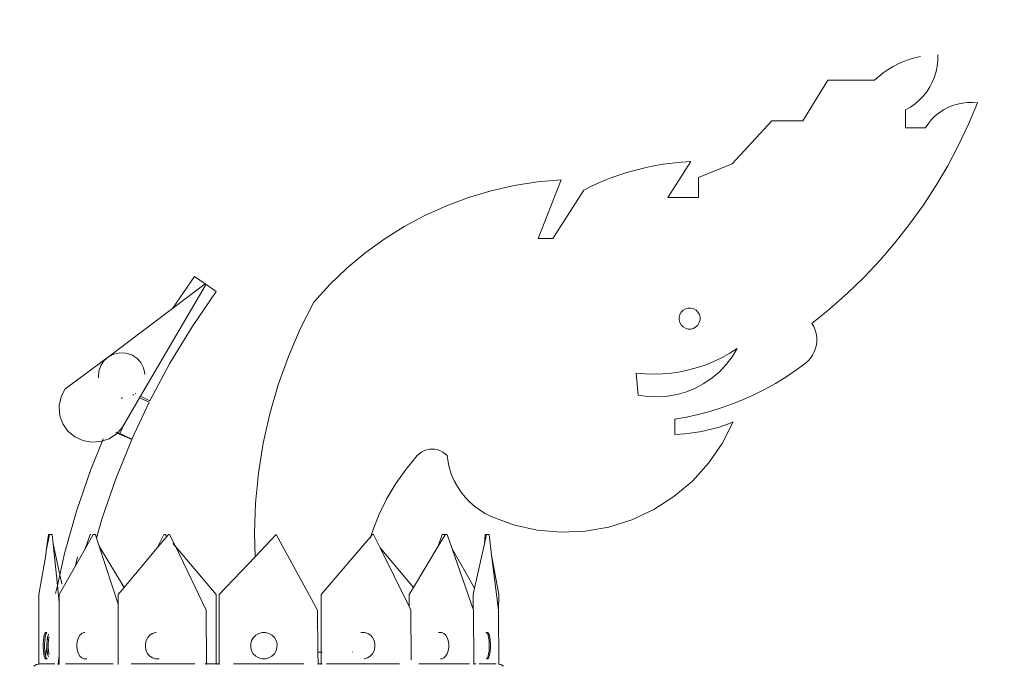
# Model space of a CAD drawing. Units: millimetres. Extents: x 7894 to 8038, y 6851 to 6951.
# Tile 40 of 49: x 7969.515 to 7972.111, y 6926.755 to 6928.457. Entities that reach past the tile are written whole.
import ezdxf

# ---------------------------------------------------------------- set-up
doc = ezdxf.new("R2010")
doc.units = ezdxf.units.MM
doc.layers.add('A-ANNO-DIMS', color=2, linetype='Continuous', lineweight=18)
doc.layers.add('A-FURN-ACCS', color=8, linetype='Continuous', lineweight=13)
doc.styles.get("Standard").update_dxf_attribs({"font": 'arial.ttf'})
doc.dimstyles.new('ISO-25', dxfattribs={"dimtxt": 1, "dimasz": 1, "dimexe": 1.25, "dimexo": 0.625, "dimtad": 1, "dimdec": 0, "dimlunit": 4, "dimtxsty": 'Standard', "dimcen": 2.5, "dimclrt": 1, "dimadec": 0, "dimazin": 0, "dimtfac": 1, "dimtdec": 0, "dimtmove": 0, "dimatfit": 3, "dimfxl": 1, "dimarcsym": 0})

# ---------------------------------------------------------------- blocks, each defined once
blk = doc.blocks.new('DISPLAY-LEAF-FINIAL-Z2_152')
for p, q in [((2.565, 3.5085, 2.1518), (2.5649, 3.4937, 2.1518)), ((2.4472, 3.4779, 2.1518), (2.4609, 3.4849, 2.1518)), ((2.4609, 3.4849, 2.1518), (2.4749, 3.4911, 2.1518)), ((2.4749, 3.4911, 2.1518), (2.4894, 3.4964, 2.1518)), ((2.4894, 3.4964, 2.1518), (2.5041, 3.5007, 2.1518)), ((2.5041, 3.5007, 2.1518), (2.5191, 3.5041, 2.1518)), ((2.5634, 3.479, 2.1518), (2.5605, 3.4646, 2.1518)), ((2.5649, 3.4937, 2.1518), (2.5634, 3.479, 2.1518)), ((2.4094, 3.4516, 2.1518), (2.4214, 3.4612, 2.1518)), ((2.4214, 3.4612, 2.1518), (2.4341, 3.4699, 2.1518)), ((2.4341, 3.4699, 2.1518), (2.4472, 3.4779, 2.1518)), ((2.5605, 3.4646, 2.1518), (2.5562, 3.4504, 2.1518)), ((2.2094, 3.3343, 2.1518), (2.2756, 3.4413, 2.1518)), ((2.2756, 3.4413, 2.1518), (2.3979, 3.4413, 2.1518)), ((2.3979, 3.4413, 2.1518), (2.4094, 3.4516, 2.1518)), ((2.5507, 3.4368, 2.1518), (2.5438, 3.4237, 2.1518)), ((2.5562, 3.4504, 2.1518), (2.5507, 3.4368, 2.1518)), ((2.5358, 3.4113, 2.1518), (2.5266, 3.3997, 2.1518)), ((2.5438, 3.4237, 2.1518), (2.5358, 3.4113, 2.1518)), ((2.5052, 3.3794, 2.1518), (2.4932, 3.3709, 2.1518)), ((2.5164, 3.3891, 2.1518), (2.5052, 3.3794, 2.1518)), ((2.5266, 3.3997, 2.1518), (2.5164, 3.3891, 2.1518)), ((2.5917, 3.3696, 2.1518), (2.604, 3.3748, 2.1518)), ((2.604, 3.3748, 2.1518), (2.6168, 3.3788, 2.1518)), ((2.6168, 3.3788, 2.1518), (2.63, 3.3815, 2.1518)), ((2.63, 3.3815, 2.1518), (2.6433, 3.3829, 2.1518)), ((2.6433, 3.3829, 2.1518), (2.6567, 3.3831, 2.1518)), ((2.6701, 3.3819, 2.1518), (2.6462, 3.3254, 2.1518)), ((2.6567, 3.3831, 2.1518), (2.6701, 3.3819, 2.1518)), ((2.4932, 3.3709, 2.1518), (2.4804, 3.3636, 2.1518)), ((2.4804, 3.3636, 2.1518), (2.4804, 3.3164, 2.1518)), ((2.5584, 3.3473, 2.1518), (2.5687, 3.3558, 2.1518)), ((2.5687, 3.3558, 2.1518), (2.5799, 3.3633, 2.1518)), ((2.5799, 3.3633, 2.1518), (2.5917, 3.3696, 2.1518)), ((2.0233, 3.2209, 2.1518), (2.1272, 3.3343, 2.1518)), ((2.1272, 3.3343, 2.1518), (2.2094, 3.3343, 2.1518)), ((2.5329, 3.3164, 2.1518), (2.5403, 3.3275, 2.1518)), ((2.5403, 3.3275, 2.1518), (2.5489, 3.3378, 2.1518)), ((2.5489, 3.3378, 2.1518), (2.5584, 3.3473, 2.1518)), ((2.6462, 3.3254, 2.1518), (2.6199, 3.27, 2.1518)), ((2.4804, 3.3164, 2.1518), (2.5329, 3.3164, 2.1518)), ((2.6199, 3.27, 2.1518), (2.5912, 3.2159, 2.1518)), ((1.8166, 3.2158, 2.1518), (1.8408, 3.2199, 2.1518)), ((1.8408, 3.2199, 2.1518), (1.8651, 3.2232, 2.1518)), ((1.9139, 3.2271, 2.1518), (1.8536, 3.1329, 2.1518)), ((1.8651, 3.2232, 2.1518), (1.8895, 3.2256, 2.1518)), ((1.8895, 3.2256, 2.1518), (1.9139, 3.2271, 2.1518)), ((1.934, 3.1854, 2.1518), (2.0233, 3.2209, 2.1518)), ((1.7219, 3.1906, 2.1518), (1.7452, 3.1982, 2.1518)), ((1.7452, 3.1982, 2.1518), (1.7688, 3.2049, 2.1518)), ((1.7688, 3.2049, 2.1518), (1.7926, 3.2108, 2.1518)), ((1.7926, 3.2108, 2.1518), (1.8166, 3.2158, 2.1518)), ((2.5912, 3.2159, 2.1518), (2.56, 3.1631, 2.1518)), ((1.4486, 3.1639, 2.1518), (1.5102, 3.1734, 2.1518)), ((1.5102, 3.1734, 2.1518), (1.5723, 3.1787, 2.1518)), ((1.5723, 3.1787, 2.1518), (1.5113, 3.0242, 2.1518)), ((1.6538, 3.163, 2.1518), (1.6762, 3.1731, 2.1518)), ((1.6762, 3.1731, 2.1518), (1.6989, 3.1823, 2.1518)), ((1.6989, 3.1823, 2.1518), (1.7219, 3.1906, 2.1518)), ((1.934, 3.1329, 2.1518), (1.934, 3.1854, 2.1518)), ((1.3281, 3.1326, 2.1518), (1.3879, 3.1503, 2.1518)), ((1.3879, 3.1503, 2.1518), (1.4486, 3.1639, 2.1518)), ((1.5498, 3.0242, 2.1518), (1.6318, 3.1522, 2.1518)), ((1.6318, 3.1522, 2.1518), (1.6538, 3.163, 2.1518)), ((2.56, 3.1631, 2.1518), (2.5265, 3.1117, 2.1518)), ((1.2698, 3.1109, 2.1518), (1.3281, 3.1326, 2.1518)), ((1.8536, 3.1329, 2.1518), (1.934, 3.1329, 2.1518)), ((1.213, 3.0852, 2.1518), (1.2698, 3.1109, 2.1518)), ((2.5265, 3.1117, 2.1518), (2.4908, 3.0619, 2.1518)), ((1.1581, 3.0558, 2.1518), (1.213, 3.0852, 2.1518)), ((1.1053, 3.0227, 2.1518), (1.1581, 3.0558, 2.1518)), ((2.4908, 3.0619, 2.1518), (2.4529, 3.0137, 2.1518)), ((1.0549, 2.9861, 2.1518), (1.1053, 3.0227, 2.1518)), ((1.5113, 3.0242, 2.1518), (1.5498, 3.0242, 2.1518)), ((2.4529, 3.0137, 2.1518), (2.4129, 2.9672, 2.1518)), ((1.0071, 2.9462, 2.1518), (1.0549, 2.9861, 2.1518)), ((2.4129, 2.9672, 2.1518), (2.3708, 2.9226, 2.1518)), ((0.9621, 2.9031, 2.1518), (1.0071, 2.9462, 2.1518)), ((0.6052, 2.9244, 2.1518), (0.5471, 2.8395, 2.1518)), ((0.634, 2.9046, 2.1518), (0.6052, 2.9244, 2.1518)), ((2.3708, 2.9226, 2.1518), (2.3268, 2.8799, 2.1518)), ((0.634, 2.9001, 2.1518), (0.4632, 2.6089, 2.1518)), ((0.634, 2.9046, 2.1518), (0.5471, 2.8395, 2.1518)), ((0.5989, 2.7915, 2.1518), (0.6629, 2.8848, 2.1518)), ((0.634, 2.9001, 2.1518), (0.634, 2.9046, 2.1518)), ((0.6629, 2.8848, 2.1518), (0.634, 2.9046, 2.1518)), ((0.9202, 2.857, 2.1518), (0.9621, 2.9031, 2.1518)), ((0.9202, 2.857, 2.1518), (0.8844, 2.7861, 2.1518)), ((2.3268, 2.8799, 2.1518), (2.2809, 2.8392, 2.1518)), ((0.5471, 2.8395, 2.1518), (0.379, 2.7129, 2.1518)), ((1.8849, 2.8243, 2.1518), (1.8885, 2.8306, 2.1518)), ((1.8885, 2.8306, 2.1518), (1.8937, 2.8357, 2.1518)), ((1.8937, 2.8357, 2.1518), (1.9001, 2.8393, 2.1518)), ((1.9001, 2.8393, 2.1518), (1.9071, 2.8412, 2.1518)), ((1.9071, 2.8412, 2.1518), (1.9144, 2.8411, 2.1518)), ((1.9144, 2.8411, 2.1518), (1.9215, 2.8392, 2.1518)), ((1.9215, 2.8392, 2.1518), (1.9278, 2.8355, 2.1518)), ((1.9278, 2.8355, 2.1518), (1.9329, 2.8304, 2.1518)), ((1.9329, 2.8304, 2.1518), (1.9365, 2.824, 2.1518)), ((2.2809, 2.8392, 2.1518), (2.2333, 2.8006, 2.1518)), ((1.8829, 2.8172, 2.1518), (1.8849, 2.8243, 2.1518)), ((1.8829, 2.8099, 2.1518), (1.8829, 2.8172, 2.1518)), ((1.8847, 2.8029, 2.1518), (1.8829, 2.8099, 2.1518)), ((1.9383, 2.8097, 2.1518), (1.9364, 2.8026, 2.1518)), ((1.9365, 2.824, 2.1518), (1.9384, 2.817, 2.1518)), ((1.9384, 2.817, 2.1518), (1.9383, 2.8097, 2.1518)), ((0.5406, 2.6956, 2.1518), (0.5989, 2.7915, 2.1518)), ((0.8844, 2.7861, 2.1518), (0.8529, 2.7132, 2.1518)), ((1.8884, 2.7965, 2.1518), (1.8847, 2.8029, 2.1518)), ((1.8935, 2.7913, 2.1518), (1.8884, 2.7965, 2.1518)), ((1.8998, 2.7877, 2.1518), (1.8935, 2.7913, 2.1518)), ((1.9068, 2.7857, 2.1518), (1.8998, 2.7877, 2.1518)), ((1.9141, 2.7857, 2.1518), (1.9068, 2.7857, 2.1518)), ((1.9212, 2.7876, 2.1518), (1.9141, 2.7857, 2.1518)), ((1.9275, 2.7912, 2.1518), (1.9212, 2.7876, 2.1518)), ((1.9327, 2.7963, 2.1518), (1.9275, 2.7912, 2.1518)), ((1.9364, 2.8026, 2.1518), (1.9327, 2.7963, 2.1518)), ((2.2333, 2.8006, 2.1518), (2.2382, 2.7921, 2.1518)), ((2.2382, 2.7921, 2.1518), (2.242, 2.7831, 2.1518)), ((2.242, 2.7831, 2.1518), (2.2446, 2.7737, 2.1518)), ((2.2446, 2.7737, 2.1518), (2.246, 2.7641, 2.1518)), ((2.2462, 2.7543, 2.1518), (2.2452, 2.7446, 2.1518)), ((2.246, 2.7641, 2.1518), (2.2462, 2.7543, 2.1518)), ((2.0364, 2.7343, 2.1518), (2.0167, 2.7218, 2.1518)), ((2.0364, 2.7343, 2.1518), (2.023, 2.7124, 2.1518)), ((2.2396, 2.7259, 2.1518), (2.2352, 2.7172, 2.1518)), ((2.243, 2.7351, 2.1518), (2.2396, 2.7259, 2.1518)), ((2.2452, 2.7446, 2.1518), (2.243, 2.7351, 2.1518)), ((0.379, 2.7129, 2.1518), (0.2637, 2.6275, 2.1518)), ((0.3584, 2.6897, 2.1518), (0.3671, 2.7026, 2.1518)), ((0.3671, 2.7026, 2.1518), (0.379, 2.7129, 2.1518)), ((0.379, 2.7129, 2.1518), (0.3932, 2.7199, 2.1518)), ((0.3932, 2.7199, 2.1518), (0.4088, 2.7231, 2.1518)), ((0.4088, 2.7231, 2.1518), (0.4248, 2.7223, 2.1518)), ((0.4248, 2.7223, 2.1518), (0.44, 2.7176, 2.1518)), ((0.44, 2.7176, 2.1518), (0.4533, 2.7092, 2.1518)), ((0.4533, 2.7092, 2.1518), (0.464, 2.6977, 2.1518)), ((0.8529, 2.7132, 2.1518), (0.8261, 2.6384, 2.1518)), ((1.9751, 2.7005, 2.1518), (1.9535, 2.6918, 2.1518)), ((1.9962, 2.7106, 2.1518), (1.9751, 2.7005, 2.1518)), ((2.0167, 2.7218, 2.1518), (1.9962, 2.7106, 2.1518)), ((2.023, 2.7124, 2.1518), (2.0073, 2.692, 2.1518)), ((2.2231, 2.7019, 2.1518), (2.2158, 2.6954, 2.1518)), ((2.2296, 2.7092, 2.1518), (2.2231, 2.7019, 2.1518)), ((2.2352, 2.7172, 2.1518), (2.2296, 2.7092, 2.1518)), ((0.3526, 2.6596, 2.1518), (0.3535, 2.675, 2.1518)), ((0.3535, 2.675, 2.1518), (0.3584, 2.6897, 2.1518)), ((0.464, 2.6977, 2.1518), (0.4713, 2.6839, 2.1518)), ((0.4713, 2.6839, 2.1518), (0.4746, 2.6689, 2.1518)), ((0.5406, 2.6956, 2.1518), (0.4875, 2.5967, 2.1518)), ((1.9089, 2.6781, 2.1518), (1.886, 2.6733, 2.1518)), ((1.9314, 2.6843, 2.1518), (1.9089, 2.6781, 2.1518)), ((1.9535, 2.6918, 2.1518), (1.9314, 2.6843, 2.1518)), ((2.0073, 2.692, 2.1518), (1.9895, 2.6734, 2.1518)), ((2.1904, 2.6768, 2.1518), (2.1643, 2.6592, 2.1518)), ((2.2158, 2.6954, 2.1518), (2.1904, 2.6768, 2.1518)), ((0.3527, 2.6591, 2.1518), (0.3526, 2.6596, 2.1518)), ((0.3526, 2.6569, 2.1518), (0.3527, 2.6591, 2.1518)), ((0.4745, 2.6667, 2.1518), (0.4746, 2.6689, 2.1518)), ((0.4745, 2.6667, 2.1518), (0.4746, 2.6661, 2.1518)), ((1.793, 2.6675, 2.1518), (1.7698, 2.6695, 2.1518)), ((1.7698, 2.6695, 2.1518), (1.7755, 2.6114, 2.1518)), ((1.8164, 2.6669, 2.1518), (1.793, 2.6675, 2.1518)), ((1.8397, 2.6677, 2.1518), (1.8164, 2.6669, 2.1518)), ((1.8629, 2.6698, 2.1518), (1.8397, 2.6677, 2.1518)), ((1.886, 2.6733, 2.1518), (1.8629, 2.6698, 2.1518)), ((1.9699, 2.6568, 2.1518), (1.9487, 2.6423, 2.1518)), ((1.9895, 2.6734, 2.1518), (1.9699, 2.6568, 2.1518)), ((2.1643, 2.6592, 2.1518), (2.1374, 2.6427, 2.1518)), ((0.2637, 2.6275, 2.1518), (0.2535, 2.6069, 2.1518)), ((0.8261, 2.6384, 2.1518), (0.804, 2.5622, 2.1518)), ((1.9261, 2.6302, 2.1518), (1.9023, 2.6205, 2.1518)), ((1.9487, 2.6423, 2.1518), (1.9261, 2.6302, 2.1518)), ((2.1099, 2.6273, 2.1518), (2.0818, 2.6132, 2.1518)), ((2.1374, 2.6427, 2.1518), (2.1099, 2.6273, 2.1518)), ((0.2535, 2.6069, 2.1518), (0.249, 2.5845, 2.1518)), ((0.4144, 2.6055, 2.1518), (0.4132, 2.6029, 2.1518)), ((0.4608, 2.6047, 2.1518), (0.4152, 2.527, 2.1518)), ((0.4431, 2.613, 2.1518), (0.4459, 2.6117, 2.1518)), ((0.4508, 2.6151, 2.1518), (0.4489, 2.6161, 2.1518)), ((0.4632, 2.6089, 2.1518), (0.4608, 2.6047, 2.1518)), ((0.4858, 2.593, 2.1518), (0.4608, 2.6047, 2.1518)), ((0.4632, 2.6089, 2.1518), (0.4875, 2.5967, 2.1518)), ((1.8009, 2.6079, 2.1518), (1.7755, 2.6114, 2.1518)), ((1.8266, 2.607, 2.1518), (1.8009, 2.6079, 2.1518)), ((1.8523, 2.6088, 2.1518), (1.8266, 2.607, 2.1518)), ((1.8776, 2.6133, 2.1518), (1.8523, 2.6088, 2.1518)), ((1.9023, 2.6205, 2.1518), (1.8776, 2.6133, 2.1518)), ((2.0531, 2.6002, 2.1518), (2.0239, 2.5884, 2.1518)), ((2.0818, 2.6132, 2.1518), (2.0531, 2.6002, 2.1518)), ((0.249, 2.58, 2.1518), (0.249, 2.5845, 2.1518)), ((0.249, 2.58, 2.1518), (0.2508, 2.5572, 2.1518)), ((0.4402, 2.4957, 2.1518), (0.4858, 2.593, 2.1518)), ((1.9942, 2.5779, 2.1518), (1.9641, 2.5686, 2.1518)), ((2.0239, 2.5884, 2.1518), (1.9942, 2.5779, 2.1518)), ((0.2508, 2.5572, 2.1518), (0.2586, 2.5356, 2.1518)), ((0.804, 2.5622, 2.1518), (0.7865, 2.4847, 2.1518)), ((1.9029, 2.5539, 2.1518), (1.8718, 2.5484, 2.1518)), ((1.8718, 2.5484, 2.1518), (1.8718, 2.5082, 2.1518)), ((1.9336, 2.5606, 2.1518), (1.9029, 2.5539, 2.1518)), ((1.9641, 2.5686, 2.1518), (1.9336, 2.5606, 2.1518)), ((0.2586, 2.5356, 2.1518), (0.2719, 2.5167, 2.1518)), ((0.4029, 2.5132, 2.1518), (0.4152, 2.527, 2.1518)), ((0.4202, 2.5355, 2.1518), (0.4085, 2.5106, 2.1518)), ((1.9502, 2.5177, 2.1518), (1.9631, 2.5206, 2.1518)), ((1.9631, 2.5206, 2.1518), (1.9758, 2.5239, 2.1518)), ((1.9758, 2.5239, 2.1518), (1.9885, 2.5276, 2.1518)), ((1.9885, 2.5276, 2.1518), (2.001, 2.5317, 2.1518)), ((2.0257, 2.5409, 2.1518), (1.9968, 2.4843, 2.1518)), ((2.001, 2.5317, 2.1518), (2.0134, 2.5361, 2.1518)), ((2.0134, 2.5361, 2.1518), (2.0257, 2.5409, 2.1518)), ((0.2719, 2.5167, 2.1518), (0.2898, 2.5018, 2.1518)), ((0.2898, 2.5018, 2.1518), (0.3111, 2.4919, 2.1518)), ((0.3628, 2.4909, 2.1518), (0.3802, 2.4968, 2.1518)), ((0.3649, 2.4962, 2.1518), (0.3628, 2.4909, 2.1518)), ((0.3802, 2.4968, 2.1518), (0.3998, 2.5097, 2.1518)), ((0.3978, 2.391, 2.1518), (0.4399, 2.4951, 2.1518)), ((0.3983, 2.5132, 2.1518), (0.4016, 2.5117, 2.1518)), ((0.3998, 2.5097, 2.1518), (0.4016, 2.5117, 2.1518)), ((0.4029, 2.5132, 2.1518), (0.4003, 2.5144, 2.1518)), ((0.4016, 2.5117, 2.1518), (0.4029, 2.5132, 2.1518)), ((0.4016, 2.5117, 2.1518), (0.4399, 2.4951, 2.1518)), ((0.4029, 2.5132, 2.1518), (0.4402, 2.4957, 2.1518)), ((0.4085, 2.5106, 2.1518), (0.4078, 2.509, 2.1518)), ((1.8718, 2.5082, 2.1518), (1.885, 2.5088, 2.1518)), ((1.885, 2.5088, 2.1518), (1.8981, 2.5098, 2.1518)), ((1.8981, 2.5098, 2.1518), (1.9112, 2.5112, 2.1518)), ((1.9112, 2.5112, 2.1518), (1.9243, 2.513, 2.1518)), ((1.9243, 2.513, 2.1518), (1.9373, 2.5152, 2.1518)), ((1.9373, 2.5152, 2.1518), (1.9502, 2.5177, 2.1518)), ((0.3111, 2.4919, 2.1518), (0.3343, 2.4876, 2.1518)), ((0.3628, 2.4909, 2.1518), (0.3323, 2.4155, 2.1518)), ((0.3343, 2.4876, 2.1518), (0.3579, 2.4893, 2.1518)), ((0.3579, 2.4893, 2.1518), (0.3628, 2.4909, 2.1518)), ((0.7865, 2.4847, 2.1518), (0.774, 2.4062, 2.1518)), ((1.2175, 2.4675, 2.1518), (1.2106, 2.465, 2.1518)), ((1.2247, 2.469, 2.1518), (1.2175, 2.4675, 2.1518)), ((1.2321, 2.4695, 2.1518), (1.2247, 2.469, 2.1518)), ((1.2395, 2.469, 2.1518), (1.2321, 2.4695, 2.1518)), ((1.2467, 2.4675, 2.1518), (1.2395, 2.469, 2.1518)), ((1.2536, 2.465, 2.1518), (1.2467, 2.4675, 2.1518)), ((1.9968, 2.4843, 2.1518), (1.9607, 2.4321, 2.1518)), ((1.1928, 2.4521, 2.1518), (1.1631, 2.4165, 2.1518)), ((1.1981, 2.4572, 2.1518), (1.1928, 2.4521, 2.1518)), ((1.2041, 2.4615, 2.1518), (1.1981, 2.4572, 2.1518)), ((1.2106, 2.465, 2.1518), (1.2041, 2.4615, 2.1518)), ((1.2601, 2.4615, 2.1518), (1.2536, 2.465, 2.1518)), ((1.2661, 2.4572, 2.1518), (1.2601, 2.4615, 2.1518)), ((1.2714, 2.4521, 2.1518), (1.2661, 2.4572, 2.1518)), ((1.274, 2.435, 2.1518), (1.2714, 2.4521, 2.1518)), ((0.3323, 2.4155, 2.1518), (0.2946, 2.3057, 2.1518)), ((1.1631, 2.4165, 2.1518), (1.1364, 2.3788, 2.1518)), ((1.278, 2.4183, 2.1518), (1.274, 2.435, 2.1518)), ((1.2834, 2.4019, 2.1518), (1.278, 2.4183, 2.1518)), ((1.9607, 2.4321, 2.1518), (1.918, 2.3851, 2.1518)), ((0.3614, 2.2848, 2.1518), (0.3978, 2.391, 2.1518)), ((0.774, 2.4062, 2.1518), (0.7662, 2.3272, 2.1518)), ((1.2903, 2.3861, 2.1518), (1.2834, 2.4019, 2.1518)), ((1.1364, 2.3788, 2.1518), (1.1127, 2.339, 2.1518)), ((1.2985, 2.371, 2.1518), (1.2903, 2.3861, 2.1518)), ((1.308, 2.3566, 2.1518), (1.2985, 2.371, 2.1518)), ((1.918, 2.3851, 2.1518), (1.8695, 2.3441, 2.1518)), ((1.1127, 2.339, 2.1518), (1.0923, 2.2975, 2.1518)), ((1.3187, 2.3431, 2.1518), (1.308, 2.3566, 2.1518)), ((1.3305, 2.3306, 2.1518), (1.3187, 2.3431, 2.1518)), ((1.8695, 2.3441, 2.1518), (1.8161, 2.3099, 2.1518)), ((0.7662, 2.3272, 2.1518), (0.7634, 2.2478, 2.1518)), ((1.3434, 2.3192, 2.1518), (1.3305, 2.3306, 2.1518)), ((1.3572, 2.3089, 2.1518), (1.3434, 2.3192, 2.1518)), ((0.2946, 2.3057, 2.1518), (0.263, 2.1941, 2.1518)), ((0.3472, 2.2349, 2.1518), (0.3614, 2.2848, 2.1518)), ((1.0923, 2.2975, 2.1518), (1.0752, 2.2545, 2.1518)), ((1.3719, 2.2999, 2.1518), (1.3572, 2.3089, 2.1518)), ((1.3873, 2.2921, 2.1518), (1.3719, 2.2999, 2.1518)), ((1.4468, 2.2701, 2.1518), (1.3873, 2.2921, 2.1518)), ((1.8161, 2.3099, 2.1518), (1.7585, 2.283, 2.1518)), ((1.5088, 2.256, 2.1518), (1.4468, 2.2701, 2.1518)), ((1.698, 2.2639, 2.1518), (1.6354, 2.2529, 2.1518)), ((1.7585, 2.283, 2.1518), (1.698, 2.2639, 2.1518)), ((0.2147, 2.201, 2.1518), (0.2202, 2.2445, 2.1518)), ((0.223, 2.2445, 2.1518), (0.2147, 2.201, 2.1518)), ((0.223, 2.2445, 2.1518), (0.2202, 2.2445, 2.1518)), ((0.223, 2.2445, 2.1518), (0.2299, 2.2445, 2.1518)), ((0.2325, 2.2195, 2.1518), (0.2299, 2.2445, 2.1518)), ((0.3171, 2.2068, 2.1518), (0.3302, 2.2445, 2.1518)), ((0.3384, 2.2445, 2.1518), (0.3171, 2.2068, 2.1518)), ((0.3318, 2.2445, 2.1518), (0.3302, 2.2445, 2.1518)), ((0.344, 2.2445, 2.1518), (0.3384, 2.2445, 2.1518)), ((0.3472, 2.2349, 2.1518), (0.344, 2.2445, 2.1518)), ((0.3543, 2.2133, 2.1518), (0.3472, 2.2349, 2.1518)), ((0.5072, 2.2093, 2.1518), (0.5246, 2.2445, 2.1518)), ((0.5322, 2.2392, 2.1518), (0.5072, 2.2093, 2.1518)), ((0.5277, 2.2445, 2.1518), (0.5246, 2.2445, 2.1518)), ((0.5277, 2.2445, 2.1518), (0.5322, 2.2392, 2.1518)), ((0.5366, 2.2445, 2.1518), (0.5322, 2.2392, 2.1518)), ((0.5399, 2.2445, 2.1518), (0.5366, 2.2445, 2.1518)), ((0.5559, 2.2114, 2.1518), (0.5399, 2.2445, 2.1518)), ((0.7634, 2.2478, 2.1518), (0.7651, 2.1857, 2.1518)), ((0.8207, 2.2445, 2.1518), (0.7651, 2.1857, 2.1518)), ((0.93, 2.0453, 2.1518), (0.8207, 2.2445, 2.1518)), ((1.0703, 2.2388, 2.1518), (0.9393, 2.0859, 2.1518)), ((1.0703, 2.2388, 2.1518), (1.069, 2.2345, 2.1518)), ((1.0707, 2.2401, 2.1518), (1.0703, 2.2388, 2.1518)), ((1.0703, 2.2388, 2.1518), (1.0715, 2.2374, 2.1518)), ((1.0752, 2.2545, 2.1518), (1.0707, 2.2401, 2.1518)), ((1.0745, 2.2445, 2.1518), (1.0707, 2.2401, 2.1518)), ((1.0745, 2.2445, 2.1518), (1.0775, 2.2445, 2.1518)), ((1.0949, 2.2093, 2.1518), (1.0775, 2.2445, 2.1518)), ((1.2478, 2.2133, 2.1518), (1.2581, 2.2445, 2.1518)), ((1.2651, 2.2421, 2.1518), (1.2478, 2.2133, 2.1518)), ((1.2581, 2.2445, 2.1518), (1.2637, 2.2445, 2.1518)), ((1.2637, 2.2445, 2.1518), (1.2651, 2.2421, 2.1518)), ((1.2666, 2.2445, 2.1518), (1.2651, 2.2421, 2.1518)), ((1.2666, 2.2445, 2.1518), (1.272, 2.2445, 2.1518)), ((1.2851, 2.2068, 2.1518), (1.272, 2.2445, 2.1518)), ((1.3696, 2.2195, 2.1518), (1.3722, 2.2445, 2.1518)), ((1.3751, 2.2445, 2.1518), (1.3696, 2.2195, 2.1518)), ((1.3722, 2.2445, 2.1518), (1.3751, 2.2445, 2.1518)), ((1.3751, 2.2445, 2.1518), (1.3819, 2.2445, 2.1518)), ((1.3819, 2.2445, 2.1518), (1.3889, 2.1901, 2.1518)), ((1.572, 2.2503, 2.1518), (1.5088, 2.256, 2.1518)), ((1.6354, 2.2529, 2.1518), (1.572, 2.2503, 2.1518)), ((0.2325, 2.2195, 2.1518), (0.2504, 2.1381, 2.1518)), ((0.2439, 2.1095, 2.1518), (0.2325, 2.2195, 2.1518)), ((0.3171, 2.2068, 2.1518), (0.2485, 2.0859, 2.1518)), ((0.3543, 2.2133, 2.1518), (0.4197, 2.1042, 2.1518)), ((0.4044, 2.0607, 2.1518), (0.3543, 2.2133, 2.1518)), ((0.5072, 2.2093, 2.1518), (0.4197, 2.1042, 2.1518)), ((0.5482, 2.2204, 2.1518), (0.5559, 2.2114, 2.1518)), ((0.5559, 2.2114, 2.1518), (0.6628, 2.0859, 2.1518)), ((0.636, 2.0453, 2.1518), (0.5559, 2.2114, 2.1518)), ((1.0949, 2.2093, 2.1518), (1.1824, 2.1042, 2.1518)), ((1.0949, 2.2093, 2.1518), (1.1714, 2.0542, 2.1518)), ((1.2478, 2.2133, 2.1518), (1.1824, 2.1042, 2.1518)), ((1.2851, 2.2068, 2.1518), (1.344, 2.1028, 2.1518)), ((1.2851, 2.2068, 2.1518), (1.3403, 2.0478, 2.1518)), ((1.3696, 2.2195, 2.1518), (1.344, 2.1028, 2.1518)), ((0.2133, 2.1901, 2.1518), (0.1946, 2.0859, 2.1518)), ((0.2133, 2.1901, 2.1518), (0.2147, 2.201, 2.1518)), ((0.263, 2.1941, 2.1518), (0.2504, 2.1381, 2.1518)), ((0.2969, 2.1855, 2.1518), (0.2915, 2.1618, 2.1518)), ((0.7651, 2.1857, 2.1518), (0.6705, 2.0859, 2.1518)), ((1.3889, 2.1901, 2.1518), (1.4075, 2.0859, 2.1518)), ((1.4073, 2.0453, 2.1518), (1.3889, 2.1901, 2.1518)), ((0.2504, 2.1381, 2.1518), (0.2439, 2.1095, 2.1518)), ((0.2504, 2.1381, 2.1518), (0.2555, 2.1145, 2.1518)), ((0.2439, 2.1095, 2.1518), (0.2392, 2.0887, 2.1518)), ((0.2485, 2.0654, 2.1518), (0.2439, 2.1095, 2.1518)), ((0.4197, 2.1042, 2.1518), (0.4044, 2.0859, 2.1518)), ((1.1824, 2.1042, 2.1518), (1.1714, 2.0859, 2.1518)), ((1.344, 2.1028, 2.1518), (1.3403, 2.0859, 2.1518)), ((0.1946, 2.0859, 2.1518), (0.1952, 2.0478, 2.1518)), ((0.2485, 2.0859, 2.1518), (0.2485, 2.0654, 2.1518)), ((0.4044, 2.0859, 2.1518), (0.4044, 2.0607, 2.1518)), ((0.6628, 2.0859, 2.1518), (0.6628, 1.9035, 2.1518)), ((0.6705, 2.0859, 2.1518), (0.6705, 1.9035, 2.1518)), ((0.9393, 2.0859, 2.1518), (0.9393, 1.9343, 2.1518)), ((1.1714, 2.0859, 2.1518), (1.1714, 2.0542, 2.1518)), ((1.3403, 2.0859, 2.1518), (1.3403, 2.0478, 2.1518)), ((1.4075, 2.0859, 2.1518), (1.4073, 2.0453, 2.1518)), ((0.2485, 2.0654, 2.1518), (0.2485, 1.9035, 2.1518)), ((0.4044, 2.0607, 2.1518), (0.4044, 1.9015, 2.1518)), ((1.1758, 2.0453, 2.1518), (1.1714, 2.0542, 2.1518)), ((0.1949, 2.0453, 2.1518), (0.1946, 1.903, 2.1518)), ((0.1949, 2.0453, 2.1518), (0.1952, 2.0478, 2.1518)), ((0.636, 2.0453, 2.1518), (0.6371, 1.9035, 2.1518)), ((0.93, 2.0453, 2.1518), (0.9309, 1.9342, 2.1518)), ((1.1758, 2.0453, 2.1518), (1.1768, 1.9142, 2.1518)), ((1.3412, 2.0453, 2.1518), (1.3403, 2.0478, 2.1518)), ((1.3412, 2.0453, 2.1518), (1.3419, 1.9035, 2.1518)), ((1.4073, 2.0453, 2.1518), (1.4075, 1.903, 2.1518)), ((0.2082, 1.9727, 2.1518), (0.2095, 1.9791, 2.1518)), ((0.2095, 1.9791, 2.1518), (0.211, 1.9837, 2.1518)), ((0.211, 1.9837, 2.1518), (0.2126, 1.986, 2.1518)), ((0.2117, 1.9727, 2.1518), (0.2129, 1.9791, 2.1518)), ((0.2161, 1.986, 2.1518), (0.2126, 1.986, 2.1518)), ((0.2129, 1.9791, 2.1518), (0.2144, 1.9837, 2.1518)), ((0.2144, 1.9837, 2.1518), (0.2161, 1.986, 2.1518)), ((0.2194, 1.979, 2.1518), (0.2179, 1.9725, 2.1518)), ((0.2202, 1.9812, 2.1518), (0.2194, 1.979, 2.1518)), ((0.2204, 1.9806, 2.1518), (0.2194, 1.979, 2.1518)), ((0.2218, 1.9746, 2.1518), (0.2213, 1.9725, 2.1518)), ((0.2996, 1.9727, 2.1518), (0.3035, 1.9791, 2.1518)), ((0.3035, 1.9791, 2.1518), (0.3083, 1.9837, 2.1518)), ((0.3083, 1.9837, 2.1518), (0.3135, 1.986, 2.1518)), ((0.3163, 1.986, 2.1518), (0.3135, 1.986, 2.1518)), ((0.482, 1.9727, 2.1518), (0.4877, 1.9791, 2.1518)), ((0.4877, 1.9791, 2.1518), (0.4947, 1.9837, 2.1518)), ((0.4947, 1.9837, 2.1518), (0.5025, 1.986, 2.1518)), ((0.5041, 1.986, 2.1518), (0.5025, 1.986, 2.1518)), ((0.7606, 1.9727, 2.1518), (0.7671, 1.9791, 2.1518)), ((0.7671, 1.9791, 2.1518), (0.775, 1.9837, 2.1518)), ((0.775, 1.9837, 2.1518), (0.7838, 1.986, 2.1518)), ((0.7838, 1.986, 2.1518), (0.7929, 1.986, 2.1518)), ((0.7929, 1.986, 2.1518), (0.8018, 1.9836, 2.1518)), ((0.8018, 1.9836, 2.1518), (0.8096, 1.979, 2.1518)), ((0.8096, 1.979, 2.1518), (0.8161, 1.9725, 2.1518)), ((1.0443, 1.986, 2.1518), (1.0459, 1.986, 2.1518)), ((1.0459, 1.986, 2.1518), (1.0541, 1.986, 2.1518)), ((1.0541, 1.986, 2.1518), (1.062, 1.9836, 2.1518)), ((1.062, 1.9836, 2.1518), (1.0691, 1.979, 2.1518)), ((1.0691, 1.979, 2.1518), (1.0749, 1.9725, 2.1518)), ((1.2486, 1.986, 2.1518), (1.2513, 1.986, 2.1518)), ((1.2513, 1.986, 2.1518), (1.2571, 1.986, 2.1518)), ((1.2571, 1.986, 2.1518), (1.2627, 1.9836, 2.1518)), ((1.2627, 1.9836, 2.1518), (1.2677, 1.979, 2.1518)), ((1.2677, 1.979, 2.1518), (1.2717, 1.9725, 2.1518)), ((1.3734, 1.986, 2.1518), (1.3755, 1.986, 2.1518)), ((1.3755, 1.986, 2.1518), (1.3775, 1.9836, 2.1518)), ((1.3755, 1.986, 2.1518), (1.3768, 1.986, 2.1518)), ((1.3768, 1.986, 2.1518), (1.3789, 1.986, 2.1518)), ((1.3775, 1.9836, 2.1518), (1.3794, 1.979, 2.1518)), ((1.3789, 1.986, 2.1518), (1.3809, 1.9836, 2.1518)), ((1.3794, 1.979, 2.1518), (1.3809, 1.9725, 2.1518)), ((1.3809, 1.9836, 2.1518), (1.3828, 1.979, 2.1518)), ((1.3828, 1.979, 2.1518), (1.3843, 1.9725, 2.1518)), ((0.2069, 1.956, 2.1518), (0.2074, 1.9648, 2.1518)), ((0.2069, 1.9469, 2.1518), (0.2069, 1.956, 2.1518)), ((0.2074, 1.9648, 2.1518), (0.2082, 1.9727, 2.1518)), ((0.2103, 1.956, 2.1518), (0.2108, 1.9648, 2.1518)), ((0.2103, 1.9469, 2.1518), (0.2103, 1.956, 2.1518)), ((0.2108, 1.9648, 2.1518), (0.2117, 1.9727, 2.1518)), ((0.2168, 1.9646, 2.1518), (0.2163, 1.9558, 2.1518)), ((0.2163, 1.9558, 2.1518), (0.2163, 1.9467, 2.1518)), ((0.2179, 1.9725, 2.1518), (0.2168, 1.9646, 2.1518)), ((0.218, 1.9665, 2.1518), (0.2168, 1.9646, 2.1518)), ((0.2179, 1.9725, 2.1518), (0.218, 1.9665, 2.1518)), ((0.2202, 1.9646, 2.1518), (0.2197, 1.9558, 2.1518)), ((0.2197, 1.9558, 2.1518), (0.2197, 1.9467, 2.1518)), ((0.2213, 1.9725, 2.1518), (0.2202, 1.9646, 2.1518)), ((0.2955, 1.956, 2.1518), (0.2969, 1.9648, 2.1518)), ((0.2955, 1.9469, 2.1518), (0.2955, 1.956, 2.1518)), ((0.2969, 1.9648, 2.1518), (0.2996, 1.9727, 2.1518)), ((0.4759, 1.956, 2.1518), (0.478, 1.9648, 2.1518)), ((0.4759, 1.9469, 2.1518), (0.4759, 1.956, 2.1518)), ((0.478, 1.9648, 2.1518), (0.482, 1.9727, 2.1518)), ((0.7536, 1.956, 2.1518), (0.756, 1.9648, 2.1518)), ((0.7536, 1.9469, 2.1518), (0.7536, 1.956, 2.1518)), ((0.756, 1.9648, 2.1518), (0.7606, 1.9727, 2.1518)), ((0.8161, 1.9725, 2.1518), (0.8206, 1.9646, 2.1518)), ((0.8206, 1.9646, 2.1518), (0.823, 1.9558, 2.1518)), ((0.823, 1.9558, 2.1518), (0.8229, 1.9467, 2.1518)), ((1.0749, 1.9725, 2.1518), (1.079, 1.9646, 2.1518)), ((1.079, 1.9646, 2.1518), (1.0811, 1.9558, 2.1518)), ((1.0811, 1.9558, 2.1518), (1.081, 1.9467, 2.1518)), ((1.2717, 1.9725, 2.1518), (1.2746, 1.9646, 2.1518)), ((1.2746, 1.9646, 2.1518), (1.2761, 1.9558, 2.1518)), ((1.2761, 1.9558, 2.1518), (1.2761, 1.9467, 2.1518)), ((1.3809, 1.9725, 2.1518), (1.3819, 1.9646, 2.1518)), ((1.3819, 1.9646, 2.1518), (1.3825, 1.9558, 2.1518)), ((1.3825, 1.9558, 2.1518), (1.3824, 1.9467, 2.1518)), ((1.3843, 1.9725, 2.1518), (1.3853, 1.9646, 2.1518)), ((1.3853, 1.9646, 2.1518), (1.3859, 1.9558, 2.1518)), ((1.3859, 1.9558, 2.1518), (1.3858, 1.9467, 2.1518)), ((0.2073, 1.938, 2.1518), (0.2069, 1.9469, 2.1518)), ((0.2082, 1.9301, 2.1518), (0.2073, 1.938, 2.1518)), ((0.2094, 1.9237, 2.1518), (0.2082, 1.9301, 2.1518)), ((0.2109, 1.9191, 2.1518), (0.2094, 1.9237, 2.1518)), ((0.2108, 1.938, 2.1518), (0.2103, 1.9469, 2.1518)), ((0.2116, 1.9301, 2.1518), (0.2108, 1.938, 2.1518)), ((0.2129, 1.9237, 2.1518), (0.2116, 1.9301, 2.1518)), ((0.2163, 1.9467, 2.1518), (0.2129, 1.9237, 2.1518)), ((0.2143, 1.9191, 2.1518), (0.2129, 1.9237, 2.1518)), ((0.2163, 1.9467, 2.1518), (0.2168, 1.9379, 2.1518)), ((0.2168, 1.9379, 2.1518), (0.2179, 1.93, 2.1518)), ((0.2179, 1.93, 2.1518), (0.2194, 1.9235, 2.1518)), ((0.2194, 1.9235, 2.1518), (0.2202, 1.9215, 2.1518)), ((0.2197, 1.9467, 2.1518), (0.2202, 1.9379, 2.1518)), ((0.2202, 1.9379, 2.1518), (0.2213, 1.93, 2.1518)), ((0.2213, 1.93, 2.1518), (0.2218, 1.928, 2.1518)), ((0.2485, 1.9251, 2.1518), (0.2458, 1.9015, 2.1518)), ((0.2969, 1.938, 2.1518), (0.2955, 1.9469, 2.1518)), ((0.2996, 1.9301, 2.1518), (0.2969, 1.938, 2.1518)), ((0.3034, 1.9237, 2.1518), (0.2996, 1.9301, 2.1518)), ((0.3082, 1.9191, 2.1518), (0.3034, 1.9237, 2.1518)), ((0.4779, 1.938, 2.1518), (0.4759, 1.9469, 2.1518)), ((0.4819, 1.9301, 2.1518), (0.4779, 1.938, 2.1518)), ((0.4876, 1.9237, 2.1518), (0.4819, 1.9301, 2.1518)), ((0.4945, 1.9191, 2.1518), (0.4876, 1.9237, 2.1518)), ((0.756, 1.938, 2.1518), (0.7536, 1.9469, 2.1518)), ((0.7605, 1.9301, 2.1518), (0.756, 1.938, 2.1518)), ((0.7669, 1.9237, 2.1518), (0.7605, 1.9301, 2.1518)), ((0.7748, 1.9191, 2.1518), (0.7669, 1.9237, 2.1518)), ((0.8095, 1.9235, 2.1518), (0.8016, 1.919, 2.1518)), ((0.816, 1.93, 2.1518), (0.8095, 1.9235, 2.1518)), ((0.8205, 1.9379, 2.1518), (0.816, 1.93, 2.1518)), ((0.8229, 1.9467, 2.1518), (0.8205, 1.9379, 2.1518)), ((0.9393, 1.9343, 2.1518), (0.9309, 1.9342, 2.1518)), ((0.9309, 1.9342, 2.1518), (0.9312, 1.9035, 2.1518)), ((0.9424, 1.9343, 2.1518), (0.9393, 1.9343, 2.1518)), ((0.9393, 1.9343, 2.1518), (0.9393, 1.9035, 2.1518)), ((1.0224, 1.935, 2.1518), (1.0208, 1.935, 2.1518)), ((1.069, 1.9235, 2.1518), (1.0618, 1.919, 2.1518)), ((1.0748, 1.93, 2.1518), (1.069, 1.9235, 2.1518)), ((1.0789, 1.9379, 2.1518), (1.0748, 1.93, 2.1518)), ((1.081, 1.9467, 2.1518), (1.0789, 1.9379, 2.1518)), ((1.2676, 1.9235, 2.1518), (1.2626, 1.919, 2.1518)), ((1.2717, 1.93, 2.1518), (1.2676, 1.9235, 2.1518)), ((1.2746, 1.9379, 2.1518), (1.2717, 1.93, 2.1518)), ((1.2761, 1.9467, 2.1518), (1.2746, 1.9379, 2.1518)), ((1.3793, 1.9235, 2.1518), (1.3775, 1.919, 2.1518)), ((1.3808, 1.93, 2.1518), (1.3793, 1.9235, 2.1518)), ((1.3819, 1.9379, 2.1518), (1.3808, 1.93, 2.1518)), ((1.3827, 1.9235, 2.1518), (1.3809, 1.919, 2.1518)), ((1.3824, 1.9467, 2.1518), (1.3819, 1.9379, 2.1518)), ((1.3842, 1.93, 2.1518), (1.3827, 1.9235, 2.1518)), ((1.3853, 1.9379, 2.1518), (1.3842, 1.93, 2.1518)), ((1.3858, 1.9467, 2.1518), (1.3853, 1.9379, 2.1518)), ((0.1817, 1.8976, 2.1518), (0.1886, 1.9015, 2.1518)), ((0.1886, 1.9015, 2.1518), (0.1946, 1.903, 2.1518)), ((0.1946, 1.903, 2.1518), (0.1964, 1.9035, 2.1518)), ((0.1946, 1.903, 2.1518), (0.1946, 1.9015, 2.1518)), ((0.1964, 1.9035, 2.1518), (0.1977, 1.9034, 2.1518)), ((0.1964, 1.9035, 2.1518), (0.1969, 1.9035, 2.1518)), ((0.2373, 1.9035, 2.1518), (0.1977, 1.9034, 2.1518)), ((0.2126, 1.9167, 2.1518), (0.2109, 1.9191, 2.1518)), ((0.2143, 1.9167, 2.1518), (0.2126, 1.9167, 2.1518)), ((0.216, 1.9167, 2.1518), (0.2143, 1.9191, 2.1518)), ((0.216, 1.9167, 2.1518), (0.2143, 1.9167, 2.1518)), ((0.2177, 1.9167, 2.1518), (0.216, 1.9167, 2.1518)), ((0.2485, 1.9035, 2.1518), (0.2439, 1.9035, 2.1518)), ((0.2485, 1.9035, 2.1518), (0.2485, 1.9015, 2.1518)), ((0.3912, 1.9035, 2.1518), (0.265, 1.9035, 2.1518)), ((0.3134, 1.9167, 2.1518), (0.3082, 1.9191, 2.1518)), ((0.3189, 1.9167, 2.1518), (0.3134, 1.9167, 2.1518)), ((0.3217, 1.9167, 2.1518), (0.3189, 1.9167, 2.1518)), ((0.4385, 1.9035, 2.1518), (0.6066, 1.9035, 2.1518)), ((0.5023, 1.9167, 2.1518), (0.4945, 1.9191, 2.1518)), ((0.5103, 1.9167, 2.1518), (0.5023, 1.9167, 2.1518)), ((0.512, 1.9167, 2.1518), (0.5103, 1.9167, 2.1518)), ((0.6371, 1.9035, 2.1518), (0.6338, 1.9035, 2.1518)), ((0.6371, 1.9035, 2.1518), (0.6371, 1.9015, 2.1518)), ((0.6628, 1.9035, 2.1518), (0.6371, 1.9035, 2.1518)), ((0.6628, 1.9035, 2.1518), (0.6705, 1.9035, 2.1518)), ((0.6628, 1.9035, 2.1518), (0.6628, 1.9015, 2.1518)), ((0.6705, 1.9035, 2.1518), (0.6705, 1.9015, 2.1518)), ((0.7081, 1.9035, 2.1518), (0.894, 1.9035, 2.1518)), ((0.7836, 1.9167, 2.1518), (0.7748, 1.9191, 2.1518)), ((0.7928, 1.9167, 2.1518), (0.7836, 1.9167, 2.1518)), ((0.8016, 1.919, 2.1518), (0.7928, 1.9167, 2.1518)), ((0.9312, 1.9035, 2.1518), (0.9312, 1.9015, 2.1518)), ((0.9393, 1.9035, 2.1518), (0.9312, 1.9035, 2.1518)), ((0.9424, 1.9035, 2.1518), (0.9393, 1.9035, 2.1518)), ((0.9393, 1.9035, 2.1518), (0.9393, 1.9015, 2.1518)), ((0.9534, 1.9035, 2.1518), (1.1456, 1.9035, 2.1518)), ((1.0524, 1.9167, 2.1518), (1.0539, 1.9167, 2.1518)), ((1.0618, 1.919, 2.1518), (1.0539, 1.9167, 2.1518)), ((1.3304, 1.9035, 2.1518), (1.1965, 1.9035, 2.1518)), ((1.2543, 1.9167, 2.1518), (1.257, 1.9167, 2.1518)), ((1.2626, 1.919, 2.1518), (1.257, 1.9167, 2.1518)), ((1.3471, 1.9035, 2.1518), (1.3419, 1.9035, 2.1518)), ((1.3419, 1.9035, 2.1518), (1.342, 1.9015, 2.1518)), ((1.3561, 1.9035, 2.1518), (1.4004, 1.9035, 2.1518)), ((1.3775, 1.919, 2.1518), (1.3755, 1.9167, 2.1518)), ((1.3755, 1.9167, 2.1518), (1.3789, 1.9167, 2.1518)), ((1.3809, 1.919, 2.1518), (1.3789, 1.9167, 2.1518)), ((1.4075, 1.903, 2.1518), (1.4135, 1.9015, 2.1518)), ((1.4075, 1.903, 2.1518), (1.4075, 1.9015, 2.1518)), ((1.4135, 1.9015, 2.1518), (1.4205, 1.8976, 2.1518))]:
    blk.add_line(p, q)
blk = doc.blocks.new('*D23')
at = {"layer": 'A-ANNO-DIMS', "color": 0, "lineweight": -2, "transparency": 16777216}
for p, q in [((7940.0888, 6907.098), (7940.0888, 6947.7928)), ((7971.9356, 6928.989), (7971.9356, 6947.7928)), ((7941.0888, 6946.5428), (7970.9356, 6946.5428))]:
    blk.add_line(p, q, dxfattribs=at)
at = {"layer": 'A-ANNO-DIMS', "color": 0, "transparency": 16777216}
for points in [[(7941.0888, 6946.7095), (7941.0888, 6946.3762), (7940.0888, 6946.5428)], [(7970.9356, 6946.7095), (7970.9356, 6946.3762), (7971.9356, 6946.5428)]]:
    blk.add_solid(points, dxfattribs=at)
at = {"layer": 'Defpoints', "color": 0, "transparency": 16777216}
for p in [(7971.9356, 6946.5428), (7971.9356, 6928.364), (7940.0888, 6906.473)]:
    blk.add_point(p, dxfattribs=at)
at = {"layer": 'A-ANNO-DIMS', "color": 1, "transparency": 16777216, "insert": (7956.0122, 6947.6784), "char_height": 1, "attachment_point": 5}
blk.add_mtext('2\'-8"', dxfattribs=at)
blk = doc.blocks.new('*D28')
at = {"layer": 'A-ANNO-DIMS', "color": 0, "lineweight": -2, "transparency": 16777216}
for p, q in [((7960.8854, 6936.8804), (7975.2272, 6936.8804)), ((7973.9772, 6935.8804), (7973.9772, 6923.6283)), ((7971.8421, 6922.6283), (7975.2272, 6922.6283))]:
    blk.add_line(p, q, dxfattribs=at)
at = {"layer": 'A-ANNO-DIMS', "color": 0, "transparency": 16777216}
for points in [[(7973.8105, 6935.8804), (7974.1439, 6935.8804), (7973.9772, 6936.8804)], [(7973.8105, 6923.6283), (7974.1439, 6923.6283), (7973.9772, 6922.6283)]]:
    blk.add_solid(points, dxfattribs=at)
at = {"layer": 'Defpoints', "color": 0, "transparency": 16777216}
for p in [(7960.2604, 6936.8804), (7971.2171, 6922.6283), (7973.9772, 6922.6283)]:
    blk.add_point(p, dxfattribs=at)
at = {"layer": 'A-ANNO-DIMS', "color": 1, "transparency": 16777216, "insert": (7972.8351, 6929.7543), "char_height": 1, "attachment_point": 5, "rotation": 90}
blk.add_mtext('1\'-2 1/2"', dxfattribs=at)

msp = doc.modelspace()

# ---------------------------------------------------------------- block references
at = {"layer": 'A-FURN-ACCS'}
msp.add_blockref('DISPLAY-LEAF-FINIAL-Z2_152', (7969.3706, 6924.8555), dxfattribs=at)

# ---------------------------------------------------------------- dimensions: what is measured, and where the dimension line sits
at = {"layer": 'A-ANNO-DIMS'}
dim = msp.add_linear_dim(base=(7971.9356, 6946.5428), p1=(7940.0888, 6906.473), p2=(7971.9356, 6928.364), dimstyle='ISO-25', override={"dimdec": 1, "dimlfac": 1, "dimrnd": 0, "dimzin": 1, "dimdsep": 46, "dimlunit": 4, "dimfrac": 2}, dxfattribs=at)
dim.commit()
dim.dimension.update_dxf_attribs({"geometry": '*D23', "text_midpoint": (7956.0122, 6947.6784)})
dim = msp.add_linear_dim(base=(7973.9772, 6922.6283), p1=(7960.2604, 6936.8804), p2=(7971.2171, 6922.6283), angle=90, dimstyle='ISO-25', override={"dimdec": 1, "dimlfac": 1, "dimrnd": 0, "dimzin": 1, "dimdsep": 46, "dimlunit": 4, "dimfrac": 2}, dxfattribs=at)
dim.commit()
dim.dimension.update_dxf_attribs({"geometry": '*D28', "text_midpoint": (7972.8351, 6929.7543)})

doc.saveas('drawing.dxf')
